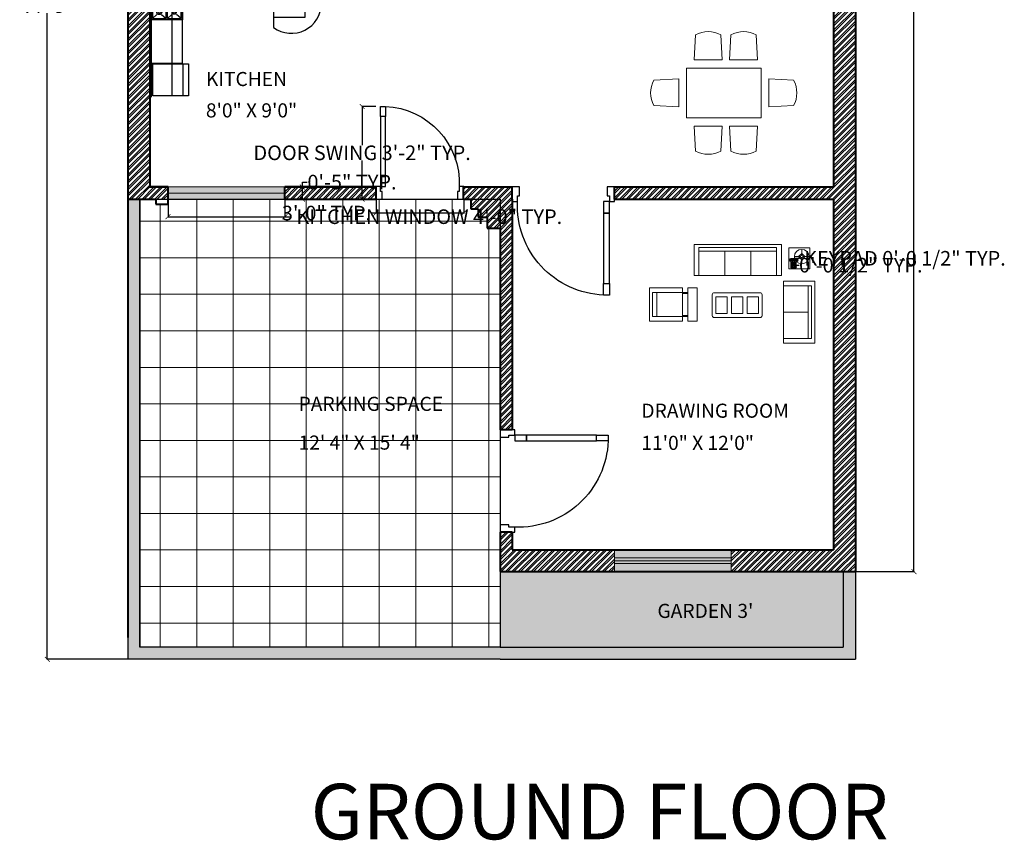
# Model space of a CAD drawing. Units: inches. Extents: x 528 to 2520, y -151 to 1354.
# Tile 1 of 41: x 542 to 947, y 706 to 1043. Entities that reach past the tile are written whole.
import ezdxf

# ---------------------------------------------------------------- set-up
doc = ezdxf.new("R2010")
doc.units = ezdxf.units.IN
doc.header["$MEASUREMENT"] = 0
for name, color, linetype, lineweight in [('A-ANNO-DIMS', 2, 'Continuous', 18), ('A-ANNO-TEXT', 7, 'Continuous', 30), ('A-AREA-IDEN', 7, 'Continuous', 18), ('A-Door', 150, 'Continuous', 25), ('A-FLOR-CASE', 11, 'Continuous', 20), ('A-FLOR-PATT', 7, 'Continuous', 13), ('A-FURN', 8, 'Continuous', 18), ('A-SITE-EDGE', 7, 'Continuous', 25), ('A-SITE-PATT', 7, 'Continuous', 13), ('A-WALL-PATT', 6, 'Continuous', 13), ('walls', 7, 'Continuous', 40), ('WINDOWS', 2, 'Continuous', 20)]:
    doc.layers.add(name, color=color, linetype=linetype, lineweight=lineweight)
doc.layers.add('A-GLAZ-PATT', color=152, linetype='Continuous', lineweight=13, true_color=0x2776bb)
doc.layers.add('L-PLNT-PATT', color=85, linetype='Continuous', lineweight=13, true_color=0x58ba48)
for name, color, linetype in [('ESYA', 11, 'Continuous'), ('NT', 1, 'Continuous'), ('TEFRIS', 11, 'Continuous')]:
    doc.layers.add(name, color=color, linetype=linetype)
doc.styles.get("Standard").update_dxf_attribs({"font": 'arial.ttf'})
doc.dimstyles.get("Standard").update_dxf_attribs({"dimtxt": 6, "dimasz": 2, "dimexe": 0.18, "dimexo": 0.0625, "dimgap": 0.09, "dimtad": 0, "dimtih": 1, "dimtoh": 1, "dimdec": 1, "dimzin": 0, "dimdsep": 46, "dimlunit": 3, "dimtxsty": 'Standard', "dimblk": 'ARCHTICK', "dimcen": 0.09, "dimadec": 0, "dimazin": 0, "dimtfac": 1, "dimtdec": 1, "dimtofl": 0, "dimtmove": 0, "dimatfit": 3, "dimfxl": 1, "dimtolj": 1, "dimtzin": 0, "dimarcsym": 0})

# ---------------------------------------------------------------- blocks, each defined once
blk = doc.blocks.new('A$C7DB75F4D')
at = {"layer": 'A-Door'}
for points in [[(625, 740), (625, 660), (665, 660), (665, 740)], [(625, 180), (625, 660), (665, 660), (665, 180)], [(625, 100), (625, 180), (665, 180), (665, 100)], [(35, 100), (35, 60), (50, 60), (50, 50), (50, 0), (0, 0), (0, 100)], [(665, 100), (700, 100), (700, 0), (650, 0), (650, 50), (650, 60), (665, 60)]]:
    blk.add_lwpolyline(points, close=True, dxfattribs=at)
at = {"layer": 'NT'}
blk.add_arc((650, 125), 615.5, 92.32782, 182.32782, dxfattribs=at)
blk = doc.blocks.new('AR365L')
blk.add_line((0, 0.1), (0.61, 0.1))
blk.add_lwpolyline([(0, 0), (0, 0.68), (0.61, 0.68), (0.61, 0)], close=True)
blk = doc.blocks.new('FIRIN1')
at = {"layer": 'ESYA'}
for p, q in [((0.288, -0.05), (0.288, -0.301)), ((0.398, -0.132), (0.312, -0.05)), ((0.575, -0.05), (0.489, -0.132)), ((0.288, -0.301), (0.025, -0.301)), ((0.025, -0.324), (0.111, -0.406)), ((0.202, -0.406), (0.288, -0.324)), ((0.398, -0.219), (0.312, -0.301)), ((0.398, -0.406), (0.312, -0.324)), ((0.575, -0.301), (0.489, -0.219)), ((0.575, -0.324), (0.489, -0.406)), ((0.025, -0.575), (0.111, -0.493)), ((0.202, -0.493), (0.288, -0.575)), ((0.398, -0.493), (0.312, -0.575)), ((0.575, -0.575), (0.489, -0.493))]:
    blk.add_line(p, q, dxfattribs=at)
blk.add_lwpolyline([(0, 0), (0.6, 0), (0.6, -0.6), (0, -0.6)], close=True, dxfattribs=at)
for points in [[(0.288, -0.05), (0.025, -0.05), (0.025, -0.301)], [(0.312, -0.05), (0.312, -0.301), (0.575, -0.301)], [(0.575, -0.301), (0.575, -0.05), (0.312, -0.05)], [(0.288, -0.575), (0.288, -0.324), (0.025, -0.324)], [(0.025, -0.324), (0.025, -0.575)], [(0.312, -0.575), (0.312, -0.324), (0.575, -0.324)], [(0.312, -0.575), (0.575, -0.575), (0.575, -0.324)], [(0.025, -0.575), (0.288, -0.575)]]:
    blk.add_lwpolyline(points, dxfattribs=at)
for centre, radius in [((0.156, -0.175), 0.0986), ((0.156, -0.175), 0.0936), ((0.444, -0.175), 0.0597), ((0.444, -0.175), 0.0294), ((0.156, -0.45), 0.0492), ((0.156, -0.45), 0.0242), ((0.444, -0.45), 0.0398), ((0.444, -0.45), 0.0196)]:
    blk.add_circle(centre, radius, dxfattribs=at)
blk = doc.blocks.new('ncvn')
for p, q in [((77868.4, -4466.7), (77868.4, -4520.7)), ((77949.4, -4466.7), (77868.4, -4466.7)), ((77949.4, -4520.7), (77949.4, -4466.7))]:
    blk.add_line(p, q)
at = {"layer": 'TEFRIS'}
for p, q in [((77783.7, -4466.7), (77783.7, -4763.4)), ((77783.7, -4466.7), (78049.5, -4466.7)), ((77902, -4516.6), (77902, -4471.6)), ((78049.5, -4466.7), (78049.5, -4553.6)), ((77819.7, -4502.8), (77819.7, -4759.2)), ((77819.7, -4502.8), (78049.5, -4502.8)), ((77837.7, -4520.8), (77837.7, -4704.7)), ((77837.7, -4520.8), (77995.5, -4520.8)), ((77868.4, -4520.7), (77949.4, -4520.7)), ((77995.5, -4520.8), (77995.5, -4643)), ((78049.5, -4555), (78049.5, -4625.7)), ((78049.5, -4625.7), (77995.8, -4625.7)), ((77783.7, -4704.7), (77837.7, -4704.7))]:
    blk.add_line(p, q, dxfattribs=at)
for points in [[(77868.4, -4466.7), (77868.4, -4520.7), (77949.4, -4520.7), (77949.4, -4466.7)], [(77871.4, -4471.6), (77871.4, -4516.6), (77947, -4516.6), (77947, -4471.6)]]:
    blk.add_lwpolyline(points, close=True, dxfattribs=at)
for points in [[(77911.5, -4488.6), (77925, -4475, -1), (77926.3, -4476.3), (77912.7, -4489.8, -1)], [(77906, -4486.7), (77906, -4507.2, 0.414214), (77911.4, -4512.6), (77937.6, -4512.6, 0.414214), (77943, -4507.2), (77943, -4486.7, 0.414214), (77937.6, -4481.3), (77911.4, -4481.3, 0.414214)], [(77906.5, -4486.7), (77906.5, -4507.2, 0.414214), (77911.4, -4512.1), (77937.6, -4512.1, 0.414214), (77942.4, -4507.2), (77942.4, -4486.7, 0.414214), (77937.6, -4481.9), (77911.4, -4481.9, 0.414214)], [(77913.5, -4476.3), (77919.7, -4476.3, -0.563183), (77919.7, -4477.4), (77913.5, -4477.4, -1)], [(77935.3, -4476.3), (77929.2, -4476.3, 0.563183), (77929.2, -4477.4), (77935.3, -4477.4, 1)]]:
    blk.add_lwpolyline(points, format="xyb", close=True, dxfattribs=at)
for points in [[(77873.2, -4477.9), (77900.2, -4477.9, -1), (77900.2, -4479.7), (77873.2, -4479.7, -1), (77873.2, -4477.9)], [(77873.2, -4480.6), (77900.2, -4480.6, -1), (77900.2, -4482.4), (77873.2, -4482.4, -1), (77873.2, -4480.6)], [(77873.2, -4483.3), (77900.2, -4483.3, -1), (77900.2, -4485.1), (77873.2, -4485.1, -1), (77873.2, -4483.3)], [(77873.2, -4486), (77900.2, -4486, -1), (77900.2, -4487.8), (77873.2, -4487.8, -1), (77873.2, -4486)], [(77873.2, -4488.7), (77900.2, -4488.7, -1), (77900.2, -4490.5), (77873.2, -4490.5, -1), (77873.2, -4488.7)], [(77873.2, -4491.4), (77900.2, -4491.4, -1), (77900.2, -4493.2), (77873.2, -4493.2, -1), (77873.2, -4491.4)], [(77873.2, -4494.1), (77900.2, -4494.1, -1), (77900.2, -4495.9), (77873.2, -4495.9, -1), (77873.2, -4494.1)], [(77873.2, -4496.8), (77900.2, -4496.8, -1), (77900.2, -4498.6), (77873.2, -4498.6, -1), (77873.2, -4496.8)], [(77873.2, -4499.5), (77900.2, -4499.5, -1), (77900.2, -4501.3), (77873.2, -4501.3, -1), (77873.2, -4499.5)], [(77873.2, -4502.2), (77900.2, -4502.2, -1), (77900.2, -4504), (77873.2, -4504, -1), (77873.2, -4502.2)], [(77873.2, -4504.9), (77900.2, -4504.9, -1), (77900.2, -4506.7), (77873.2, -4506.7, -1), (77873.2, -4504.9)], [(77873.2, -4507.6), (77900.2, -4507.6, -1), (77900.2, -4509.4), (77873.2, -4509.4, -1), (77873.2, -4507.6)], [(77873.2, -4510.3), (77900.2, -4510.3, -1), (77900.2, -4512.1), (77873.2, -4512.1, -1), (77873.2, -4510.3)]]:
    blk.add_lwpolyline(points, format="xyb", dxfattribs=at)
for points in [[(77901.2, -4520.7), (77901.2, -4521.6), (77902.1, -4521.6), (77902.1, -4520.7)], [(77915.6, -4520.7), (77915.6, -4521.6), (77916.5, -4521.6), (77916.5, -4520.7)]]:
    blk.add_lwpolyline(points, dxfattribs=at)
for centre, radius in [((77913, -4488.3), 0.571), ((77924.9, -4498.5), 2.86)]:
    blk.add_circle(centre, radius, dxfattribs=at)
for centre, radius, start, end in [((77918.7, -4476.9), 1.71, 199.4712, 160.5288), ((77924.4, -4476.9), 1.71, 75, 195), ((77930.2, -4476.9), 1.71, 19.4712, 340.5288), ((77924.4, -4476.9), 1.71, 255, 15), ((78026.2, -4601.3), 51.8, 233.6588, 63.2671)]:
    blk.add_arc(centre, radius, start, end, dxfattribs=at)
at = {"layer": 'TEFRIS', "xscale": 90, "yscale": 90, "zscale": 90}
blk.add_blockref('FIRIN1', (77783.8, -4575.9), dxfattribs=at)
at = {"layer": 'TEFRIS', "xscale": 90, "yscale": 90, "zscale": 90, "rotation": 90}
blk.add_blockref('AR365L', (77848.2, -4760.9), dxfattribs=at)
blk = doc.blocks.new('RECLIN32')
for p, q in [((16, 0), (16, -32)), ((-11.5, -3), (11.5, -3)), ((-11.5, -32), (-11.5, -3)), ((-11.5, -7), (11.5, -7)), ((11.5, -3), (11.5, -32)), ((-11.5, -32), (-11.5, -37)), ((-10.5, -32), (-10.5, -37)), ((10.5, -32), (10.5, -37)), ((11.5, -32), (11.5, -37))]:
    blk.add_line(p, q)
blk.add_lwpolyline([(16, -32), (-16, -32), (-16, 0), (16, 0)])
blk.add_lwpolyline([(-16, -46), (-16, -37), (16, -37), (16, -46)], close=True)
blk = doc.blocks.new('LOVESET5')
for p, q in [((35.75, 0), (35.75, -30.00001)), ((-19.75, -3), (31.25, -3)), ((-19.75, -30.00001), (-19.75, -3)), ((-19.75, -6.5), (31.25, -6.5)), ((5.75, -6.5), (5.75, -30.00001)), ((31.25, -3), (31.25, -30.00001))]:
    blk.add_line(p, q)
for points in [[(35.75, -30.00001), (-24.25, -30.00001), (-24.25, 0), (24.25, 0)], [(24.25, 0), (35.75, 0)]]:
    blk.add_lwpolyline(points)
blk = doc.blocks.new('TBLEN20S')
blk.add_lwpolyline([(-10, -10), (-10, 10), (10, 10), (10, -10)], close=True)
blk = doc.blocks.new('LAMP')
for p, q in [((-1, 0), (-7, 0)), ((0, 3), (-3, 0)), ((-3, 0), (0, -3)), ((0, 7), (0, 1)), ((3, 0), (0, 3)), ((0, -3), (3, 0)), ((1, 0), (7, 0)), ((0, -1), (0, -7))]:
    blk.add_line(p, q)
for radius in [7, 1]:
    blk.add_circle((0, 0), radius)
blk = doc.blocks.new('SOFA7')
for p, q in [((-37.5, -3), (37.5, -3)), ((-37.5, -30), (-37.5, -3)), ((-37.5, -6.5), (37.5, -6.5)), ((-12.5, -6.5), (-12.5, -30)), ((12.5, -6.5), (12.5, -30)), ((37.5, -3), (37.5, -30))]:
    blk.add_line(p, q)
blk.add_lwpolyline([(-42, -30), (-42, 0), (42, 0), (42, -30)], close=True)
blk = doc.blocks.new('TBLWGLAS')
for p, q in [((-22, 0), (22, 0)), ((-24, -22), (-24, -2)), ((-20.5, -20), (-20.5, -4)), ((-20.5, -4), (-9.5, -4)), ((-9.5, -4), (-9.5, -20)), ((-5.5, -20), (-5.5, -4)), ((-5.5, -4), (5.5, -4)), ((5.5, -4), (5.5, -20)), ((9.5, -20), (9.5, -4)), ((9.5, -4), (20.5, -4)), ((20.5, -4), (20.5, -20)), ((24, -2), (24, -22)), ((22, -24), (-22, -24)), ((-9.5, -20), (-20.5, -20)), ((5.5, -20), (-5.5, -20)), ((20.5, -20), (9.5, -20))]:
    blk.add_line(p, q)
for centre, start, end in [((-22, -2), 90, 180), ((22, -2), 0, 90), ((-22, -22), 180, 270), ((22, -22), 270, 0)]:
    blk.add_arc(centre, 2, start, end)
blk = doc.blocks.new('PHONE')
for p, q in [((-3.99, 3.5), (-3.99, 2.5)), ((4.01, 3.5), (-3.99, 3.5)), ((-3.99, 2.5), (4.01, 2.5)), ((-2.49, -4.03), (-2.49, 1.92)), ((-2.02, 4.5), (2.02, 4.5)), ((-1.99, 1), (-1.99, -4)), ((2.01, 1), (-1.99, 1)), ((-1.49, 4), (-0.74, 4)), ((-1.49, 3.5), (-1.49, 4)), ((-1.49, 2), (-1.49, 2.5)), ((-0.74, 2), (-1.49, 2)), ((1.01, 0.5), (-0.99, 0.5)), ((-0.99, 0.5), (-0.99, -3.5)), ((-0.74, 4), (-0.74, 3.5)), ((-0.74, 2.5), (-0.74, 2)), ((0.76, 4), (0.76, 3.5)), ((1.51, 4), (0.76, 4)), ((0.76, 2.5), (0.76, 2)), ((0.76, 2), (1.51, 2)), ((1.01, -3.5), (1.01, 0.5)), ((1.51, 3.5), (1.51, 4)), ((1.51, 2), (1.51, 2.5)), ((2.01, -4), (2.01, 1)), ((2.51, 1.95), (2.51, -4.06)), ((4.01, 2.5), (4.01, 3.5)), ((2.04, -4.5), (-2.01, -4.5)), ((-1.99, -4), (2.01, -4)), ((-0.99, -3.5), (1.01, -3.5))]:
    blk.add_line(p, q)
for centre, radius, start, end in [((-3.24, 3), 1.27, 24.02748, 336.6167), ((-2.05, 4.06), 0.442, 81.8699, 188.1301), ((2.07, 4.06), 0.442, 351.8699, 98.1301), ((3.26, 3), 1.25, 205.0096, 154.8206), ((-2.05, -4.06), 0.442, 171.8699, 278.1301), ((2.07, -4.06), 0.442, 261.8699, 8.1301)]:
    blk.add_arc(centre, radius, start, end)
blk = doc.blocks.new('table-20')
at = {"color": 0, "linetype": 'ByBlock'}
for p, q in [((-1.052, 0.533), (-1.074, 0.134)), ((-0.646, 0.533), (-0.624, 0.134)), ((-0.484, 0.533), (-0.506, 0.134)), ((-0.078, 0.533), (-0.056, 0.134)), ((-1.2, 0), (0, 0)), ((-1.2, -0.8), (-1.2, 0)), ((-0.624, 0.134), (-1.074, 0.134)), ((-0.056, 0.134), (-0.506, 0.134)), ((0, -0.8), (0, 0)), ((-1.723, -0.197), (-1.324, -0.175)), ((-1.324, -0.625), (-1.324, -0.175)), ((0.124, -0.625), (0.124, -0.175)), ((0.523, -0.197), (0.124, -0.175)), ((-1.723, -0.603), (-1.324, -0.625)), ((0.523, -0.603), (0.124, -0.625)), ((-1.2, -0.8), (0, -0.8)), ((-0.624, -0.934), (-1.074, -0.934)), ((-1.052, -1.333), (-1.074, -0.934)), ((-0.646, -1.333), (-0.624, -0.934)), ((-0.484, -1.333), (-0.506, -0.934)), ((-0.056, -0.934), (-0.506, -0.934)), ((-0.078, -1.333), (-0.056, -0.934))]:
    blk.add_line(p, q, dxfattribs=at)
for centre, start, end in [((-0.849, 0.159), 61.4891, 118.5109), ((-0.281, 0.159), 61.4891, 118.5109), ((-1.349, -0.4), 151.4891, 208.5109), ((0.149, -0.4), 331.4891, 28.5109), ((-0.849, -0.959), 241.4891, 298.5109), ((-0.281, -0.959), 241.4891, 298.5109)]:
    blk.add_arc(centre, 0.425, start, end, dxfattribs=at)
blk = doc.blocks.new('_ArchTick')
at = {"color": 0, "linetype": 'ByBlock', "const_width": 0.15}
blk.add_lwpolyline([(-0.5, -0.5), (0.5, 0.5)], dxfattribs=at)
blk = doc.blocks.new('*D24')
at = {"layer": 'A-ANNO-DIMS', "color": 0, "lineweight": -2, "transparency": 16777216}
for p, q in [((885.76, 1317.1), (909.9, 1317.1)), ((909.72, 1317.1), (909.72, 1069.76)), ((909.72, 816.1), (909.72, 1063.45)), ((885.76, 816.1), (909.9, 816.1))]:
    blk.add_line(p, q, dxfattribs=at)
at = {"layer": 'Defpoints', "color": 0, "transparency": 16777216}
for p in [(885.7, 1317.1), (885.7, 816.1), (909.72, 816.1)]:
    blk.add_point(p, dxfattribs=at)
at = {"layer": 'A-ANNO-DIMS', "color": 0, "lineweight": -2, "transparency": 16777216, "xscale": 2, "yscale": 2, "zscale": 2}
for p, rotation in [((909.72, 1317.1), 90), ((909.72, 816.1), 270)]:
    blk.add_blockref('_ArchTick', p, dxfattribs=dict(at, rotation=rotation))
at = {"layer": 'A-ANNO-DIMS', "color": 0, "transparency": 16777216, "insert": (909.72, 1066.6), "char_height": 6, "attachment_point": 5}
blk.add_mtext('\\A1;41\'-9.0"', dxfattribs=at)
blk = doc.blocks.new('WINDOW-48x5-PLAN')
for p, q in [((0, 5), (48, 5)), ((0, 2.5), (48, 2.5))]:
    blk.add_line(p, q)
blk.add_lwpolyline([(0, 5), (48, 5), (48, 0), (0, 0)], close=True)
blk = doc.blocks.new('WINDOW-48x9-PLAN')
for p, q in [((0, 5.63), (48, 5.63)), ((0, 4.5), (48, 4.5)), ((0, 3.37), (48, 3.37))]:
    blk.add_line(p, q)
blk.add_lwpolyline([(0, 9), (48, 9), (48, 0), (0, 0)], close=True)
blk = doc.blocks.new('TELEPHONE-KEYPAD')
for centre in [(0.05, 0.67), (0.07, 0.46), (0.09, 0.25), (0.1, 0.06), (0.26, 0.67), (0.27, 0.47), (0.27, 0.25), (0.29, 0.05), (0.48, 0.66), (0.48, 0.46), (0.49, 0.26), (0.5, 0.08)]:
    blk.add_circle(centre, 0.0493)
blk = doc.blocks.new('*D42')
at = {"layer": 'A-ANNO-DIMS', "color": 0, "lineweight": -2, "transparency": 16777216}
for p, q in [((688.64, 1007.18), (682.81, 1007.18)), ((682.99, 1007.18), (682.99, 991.34)), ((682.99, 969.1), (682.99, 984.94)), ((688.64, 969.1), (682.81, 969.1))]:
    blk.add_line(p, q, dxfattribs=at)
at = {"layer": 'Defpoints', "color": 0, "transparency": 16777216}
for p in [(682.99, 1007.18), (688.7, 1007.18), (688.7, 969.1)]:
    blk.add_point(p, dxfattribs=at)
at = {"layer": 'A-ANNO-DIMS', "color": 0, "lineweight": -2, "transparency": 16777216, "xscale": 2, "yscale": 2, "zscale": 2}
for p, rotation in [((682.99, 1007.18), 90), ((682.99, 969.1), 270)]:
    blk.add_blockref('_ArchTick', p, dxfattribs=dict(at, rotation=rotation))
at = {"layer": 'A-ANNO-DIMS', "color": 0, "transparency": 16777216, "insert": (682.99, 988.14), "char_height": 6, "attachment_point": 5}
blk.add_mtext('\\A1;DOOR SWING 3\'-2" TYP.', dxfattribs=at)
blk = doc.blocks.new('*D43')
at = {"layer": 'A-ANNO-DIMS', "color": 0, "lineweight": -2, "transparency": 16777216}
for p, q in [((688.7, 969.04), (688.7, 963.21)), ((724.72, 969.04), (724.72, 963.21)), ((688.7, 963.39), (686.7, 963.39)), ((724.72, 963.39), (688.7, 963.39))]:
    blk.add_line(p, q, dxfattribs=at)
at = {"layer": 'Defpoints', "color": 0, "transparency": 16777216}
for p in [(688.7, 969.1), (724.72, 969.1), (688.7, 963.39)]:
    blk.add_point(p, dxfattribs=at)
at = {"layer": 'A-ANNO-DIMS', "color": 0, "lineweight": -2, "transparency": 16777216, "xscale": 2, "yscale": 2, "zscale": 2, "rotation": 180}
blk.add_blockref('_ArchTick', (688.7, 963.39), dxfattribs=at)
at = {"layer": 'A-ANNO-DIMS', "color": 0, "lineweight": -2, "transparency": 16777216, "xscale": 2, "yscale": 2, "zscale": 2}
blk.add_blockref('_ArchTick', (724.72, 963.39), dxfattribs=at)
at = {"layer": 'A-ANNO-DIMS', "color": 0, "transparency": 16777216, "insert": (668.33, 963.39), "char_height": 6, "attachment_point": 5}
blk.add_mtext('\\A1;3\'-0" TYP.', dxfattribs=at)
blk = doc.blocks.new('*D76')
at = {"layer": 'A-ANNO-DIMS', "color": 0, "lineweight": -2, "transparency": 16777216}
for p, q in [((860.61, 942.81), (860.83, 942.81)), ((860.65, 942.81), (860.65, 944.81)), ((860.65, 944.81), (862.65, 944.81)), ((860.65, 942.09), (860.65, 942.81)), ((860.61, 942.09), (860.83, 942.09))]:
    blk.add_line(p, q, dxfattribs=at)
at = {"layer": 'Defpoints', "color": 0, "transparency": 16777216}
for p in [(860.54, 942.81), (860.65, 942.81), (860.54, 942.09)]:
    blk.add_point(p, dxfattribs=at)
at = {"layer": 'A-ANNO-DIMS', "color": 0, "lineweight": -2, "transparency": 16777216, "xscale": 2, "yscale": 2, "zscale": 2}
for p, rotation in [((860.65, 942.81), 90), ((860.65, 942.09), 270)]:
    blk.add_blockref('_ArchTick', p, dxfattribs=dict(at, rotation=rotation))
at = {"layer": 'A-ANNO-DIMS', "color": 0, "transparency": 16777216, "insert": (906.05, 944.81), "char_height": 6, "attachment_point": 5}
blk.add_mtext('\\A1;KEYPAD 0\'-0 1/2" TYP.', dxfattribs=at)
blk = doc.blocks.new('*D77')
at = {"layer": 'A-ANNO-DIMS', "color": 0, "lineweight": -2, "transparency": 16777216}
for p, q in [((860, 942.03), (860, 941.8)), ((860, 941.98), (860.54, 941.98)), ((860.54, 942.03), (860.54, 941.8)), ((860.54, 941.98), (862.54, 941.98))]:
    blk.add_line(p, q, dxfattribs=at)
at = {"layer": 'Defpoints', "color": 0, "transparency": 16777216}
for p in [(860, 942.09), (860.54, 942.09), (860.54, 941.98)]:
    blk.add_point(p, dxfattribs=at)
at = {"layer": 'A-ANNO-DIMS', "color": 0, "lineweight": -2, "transparency": 16777216, "xscale": 2, "yscale": 2, "zscale": 2, "rotation": 180}
blk.add_blockref('_ArchTick', (860, 941.98), dxfattribs=at)
at = {"layer": 'A-ANNO-DIMS', "color": 0, "lineweight": -2, "transparency": 16777216, "xscale": 2, "yscale": 2, "zscale": 2}
blk.add_blockref('_ArchTick', (860.54, 941.98), dxfattribs=at)
at = {"layer": 'A-ANNO-DIMS', "color": 0, "transparency": 16777216, "insert": (887.91, 941.98), "char_height": 6, "attachment_point": 5}
blk.add_mtext('\\A1;0\'-0 1/2" TYP.', dxfattribs=at)
blk = doc.blocks.new('*D84')
at = {"layer": 'A-ANNO-DIMS', "color": 0, "lineweight": -2, "transparency": 16777216}
for p, q in [((603.24, 969.04), (603.24, 961.72)), ((651.24, 969.04), (651.24, 961.72)), ((603.24, 961.9), (651.24, 961.9)), ((651.24, 961.9), (653.24, 961.9))]:
    blk.add_line(p, q, dxfattribs=at)
at = {"layer": 'Defpoints', "color": 0, "transparency": 16777216}
for p in [(603.24, 969.1), (651.24, 969.1), (651.24, 961.9)]:
    blk.add_point(p, dxfattribs=at)
at = {"layer": 'A-ANNO-DIMS', "color": 0, "lineweight": -2, "transparency": 16777216, "xscale": 2, "yscale": 2, "zscale": 2, "rotation": 180}
blk.add_blockref('_ArchTick', (603.24, 961.9), dxfattribs=at)
at = {"layer": 'A-ANNO-DIMS', "color": 0, "lineweight": -2, "transparency": 16777216, "xscale": 2, "yscale": 2, "zscale": 2}
blk.add_blockref('_ArchTick', (651.24, 961.9), dxfattribs=at)
at = {"layer": 'A-ANNO-DIMS', "color": 0, "transparency": 16777216, "insert": (710.6, 961.9), "char_height": 6, "attachment_point": 5}
blk.add_mtext('\\A1;KITCHEN WINDOW 4\'-0" TYP.', dxfattribs=at)
blk = doc.blocks.new('*D85')
at = {"layer": 'A-ANNO-DIMS', "color": 0, "lineweight": -2, "transparency": 16777216}
for p, q in [((658.44, 974.1), (658.44, 976.1)), ((658.44, 976.1), (660.44, 976.1)), ((651.31, 974.1), (658.62, 974.1)), ((658.44, 969.1), (658.44, 974.1)), ((651.31, 969.1), (658.62, 969.1))]:
    blk.add_line(p, q, dxfattribs=at)
at = {"layer": 'Defpoints', "color": 0, "transparency": 16777216}
for p in [(651.24, 974.1), (658.44, 974.1), (651.24, 969.1)]:
    blk.add_point(p, dxfattribs=at)
at = {"layer": 'A-ANNO-DIMS', "color": 0, "lineweight": -2, "transparency": 16777216, "xscale": 2, "yscale": 2, "zscale": 2}
for p, rotation in [((658.44, 974.1), 90), ((658.44, 969.1), 270)]:
    blk.add_blockref('_ArchTick', p, dxfattribs=dict(at, rotation=rotation))
at = {"layer": 'A-ANNO-DIMS', "color": 0, "transparency": 16777216, "insert": (678.82, 976.1), "char_height": 6, "attachment_point": 5}
blk.add_mtext('\\A1;0\'-5" TYP.', dxfattribs=at)
blk = doc.blocks.new('*D92')
at = {"layer": 'A-ANNO-DIMS', "color": 0, "lineweight": -2, "transparency": 16777216}
for p, q in [((586.63, 1317.1), (553.42, 1317.1)), ((553.6, 1317.1), (553.6, 1051.76)), ((553.6, 780.1), (553.6, 1045.45)), ((586.63, 780.1), (553.42, 780.1))]:
    blk.add_line(p, q, dxfattribs=at)
at = {"layer": 'Defpoints', "color": 0, "transparency": 16777216}
for p in [(553.6, 1317.1), (586.7, 1317.1), (586.7, 780.1)]:
    blk.add_point(p, dxfattribs=at)
at = {"layer": 'A-ANNO-DIMS', "color": 0, "lineweight": -2, "transparency": 16777216, "xscale": 2, "yscale": 2, "zscale": 2}
for p, rotation in [((553.6, 1317.1), 90), ((553.6, 780.1), 270)]:
    blk.add_blockref('_ArchTick', p, dxfattribs=dict(at, rotation=rotation))
at = {"layer": 'A-ANNO-DIMS', "color": 0, "transparency": 16777216, "insert": (553.6, 1048.6), "char_height": 6, "attachment_point": 5}
blk.add_mtext('\\A1;44\'-9"', dxfattribs=at)

msp = doc.modelspace()

# ---------------------------------------------------------------- hatches: boundary and pattern name
at = {"layer": 'A-FLOR-PATT', "transparency": 33554523}
h = msp.add_hatch(dxfattribs=at)
h.set_pattern_fill('NET', color=256, scale=120)
h.paths.add_polyline_path([(739.7, 957.24), (734.43, 957.24), (734.43, 961.68), (730.74, 961.68), (730.74, 965.12), (727.7, 965.12), (727.7, 969.1), (603.24, 969.1), (603.24, 967.1), (598.24, 967.1), (598.24, 969.1), (591.7, 969.1), (591.7, 785.1), (739.7, 785.1)])
at = {"layer": 'A-GLAZ-PATT'}
h = msp.add_hatch(color=256, dxfattribs=at)
h.dxf.hatch_style = 1
h.paths.add_polyline_path([(651.24, 974.1), (603.24, 974.1), (603.24, 971.6), (651.24, 971.6)])
h.paths.add_polyline_path([(651.24, 971.6), (603.24, 971.6), (603.24, 969.1), (651.24, 969.1)])
h = msp.add_hatch(color=256, dxfattribs=at)
h.dxf.hatch_style = 1
h.paths.add_polyline_path([(834.7, 825.1), (786.7, 825.1), (786.7, 821.73), (834.7, 821.73)])
h.paths.add_polyline_path([(834.7, 821.73), (786.7, 821.73), (786.7, 820.6), (834.7, 820.6)])
h.paths.add_polyline_path([(834.7, 820.6), (786.7, 820.6), (786.7, 819.47), (834.7, 819.47)])
h.paths.add_polyline_path([(834.7, 819.47), (786.7, 819.47), (786.7, 816.1), (834.7, 816.1)])
at = {"layer": 'A-SITE-PATT'}
h = msp.add_hatch(color=256, dxfattribs=at)
h.dxf.hatch_style = 1
h.paths.add_polyline_path([(885.7, 816.1), (880.7, 816.1), (880.7, 785.1), (739.7, 785.1), (591.7, 785.1), (591.7, 969.1), (586.7, 969.1), (586.7, 789.1), (586.7, 780.1), (739.7, 780.1), (885.7, 780.1)])
at = {"layer": 'A-WALL-PATT'}
h = msp.add_hatch(dxfattribs=at)
h.set_pattern_fill('ANSI32', color=256, scale=5)
h.paths.add_polyline_path([(595.7, 1163.86), (586.7, 1163.86), (586.7, 969.1), (598.24, 969.1), (603.24, 969.1), (603.24, 974.1), (595.7, 974.1), (595.7, 1082.1), (691.7, 1082.1), (691.7, 1087.1), (691.7, 1106.1), (697.7, 1106.1), (697.7, 1111.1), (686.7, 1111.1), (686.7, 1087.1), (595.7, 1087.1)])
h.paths.add_polyline_path([(688.7, 974.1), (651.24, 974.1), (651.24, 969.1), (688.7, 969.1)])
h.paths.add_polyline_path([(885.7, 1171.37), (876.7, 1171.37), (876.7, 1111.1), (786.7, 1111.1), (786.7, 1106.1), (876.7, 1106.1), (876.7, 974.1), (786.7, 974.1), (786.7, 969.1), (876.7, 969.1), (876.7, 825.1), (834.7, 825.1), (834.7, 816.1), (885.7, 816.1)])
h.paths.add_polyline_path([(885.7, 1317.1), (876.65, 1317.1), (876.65, 1308.1), (876.7, 1308.1), (876.7, 1248.1), (822.7, 1248.1), (822.7, 1243.1), (876.7, 1243.1), (876.7, 1219.37), (885.7, 1219.37)])
h.paths.add_polyline_path([(852.65, 1317.1), (787.7, 1317.1), (787.7, 1248.1), (784.26, 1248.1), (784.26, 1243.1), (792.7, 1243.1), (792.7, 1249.1), (792.7, 1308.1), (852.65, 1308.1)])
h.paths.add_polyline_path([(684.7, 1317.1), (619.7, 1317.1), (619.7, 1308.1), (679.7, 1308.1), (679.7, 1248.1), (679.7, 1243.1), (684.7, 1243.1), (684.7, 1248.25)])
h.paths.add_polyline_path([(595.7, 1308.1), (595.7, 1317.1), (586.7, 1317.1), (586.7, 1211.86), (595.7, 1211.86), (595.7, 1243.1), (649.7, 1243.1), (649.7, 1248.1), (595.7, 1248.1)])
h.paths.add_polyline_path([(744.7, 969.1), (744.7, 974.1), (724.7, 974.1), (724.7, 969.1), (739.7, 969.1), (739.7, 874.29), (744.7, 874.29)])
h.paths.add_polyline_path([(739.7, 969.1), (727.7, 969.1), (727.7, 965.12), (730.74, 965.12), (730.74, 961.68), (734.43, 961.68), (734.43, 957.24), (739.7, 957.24)], flags=17)
h.paths.add_polyline_path([(786.7, 825.1), (744.7, 825.1), (744.7, 832.29), (739.7, 832.29), (739.7, 816.1), (786.7, 816.1)])
at = {"layer": 'L-PLNT-PATT', "transparency": 33554577}
h = msp.add_hatch(color=256, dxfattribs=at)
h.dxf.hatch_style = 1
h.paths.add_polyline_path([(880.7, 816.1), (739.7, 816.1), (739.7, 785.1), (880.7, 785.1)])
h.paths.add_polyline_path([(802.83, 795.49), (848.74, 795.49), (848.74, 804.48), (802.83, 804.48)], flags=24)

# ---------------------------------------------------------------- linework, layer by layer
at = {"layer": 'A-SITE-EDGE'}
for p, q in [((591.7, 969.1), (591.7, 785.1)), ((739.7, 816.1), (739.7, 785.1)), ((880.7, 816.1), (880.7, 785.1)), ((885.7, 816.1), (885.7, 780.1)), ((586.7, 789.1), (586.7, 780.1)), ((739.7, 785.1), (591.7, 785.1)), ((739.7, 785.1), (880.7, 785.1)), ((739.7, 780.1), (586.7, 780.1)), ((739.7, 780.1), (885.7, 780.1))]:
    msp.add_line(p, q, dxfattribs=at)
msp.add_lwpolyline([(591.7, 969.1), (739.7, 969.1), (739.7, 785.1), (591.7, 785.1)], close=True, dxfattribs=at)
at = {"layer": 'walls'}
for p, q in [((586.7, 1317.1), (586.7, 789.1)), ((885.7, 1317.1), (885.7, 816.1)), ((876.7, 1106.1), (876.7, 974.1)), ((595.7, 1082.1), (595.7, 974.1)), ((595.7, 974.1), (603.24, 974.1)), ((603.24, 974.1), (595.7, 974.1)), ((603.24, 967.1), (603.24, 974.1)), ((688.7, 974.1), (651.24, 974.1)), ((651.24, 969.1), (651.24, 974.1)), ((651.24, 974.1), (688.7, 974.1)), ((688.7, 969.1), (688.7, 974.1)), ((724.7, 969.1), (724.7, 974.1)), ((724.7, 974.1), (744.7, 974.1)), ((744.7, 969.1), (744.7, 974.1)), ((786.7, 969.1), (786.7, 974.1)), ((786.7, 974.1), (876.7, 974.1)), ((586.7, 969.1), (598.24, 969.1)), ((598.24, 969.1), (598.24, 967.1)), ((598.24, 967.1), (603.24, 967.1)), ((651.24, 969.1), (688.7, 969.1)), ((724.7, 969.1), (727.7, 969.1)), ((727.7, 969.1), (727.7, 965.12)), ((744.7, 969.1), (744.7, 874.29)), ((786.7, 969.1), (876.7, 969.1)), ((876.7, 969.1), (876.7, 825.1)), ((727.7, 965.12), (730.74, 965.12)), ((730.74, 965.12), (730.74, 961.68)), ((730.74, 961.68), (734.43, 961.68)), ((734.43, 961.68), (734.43, 957.24)), ((734.43, 957.24), (739.7, 957.24)), ((739.7, 957.24), (739.7, 874.29)), ((744.7, 874.29), (739.7, 874.29)), ((744.7, 832.29), (739.7, 832.29)), ((739.7, 832.29), (739.7, 816.1)), ((744.7, 832.29), (744.7, 825.1)), ((744.7, 825.1), (876.7, 825.1)), ((739.7, 816.1), (885.7, 816.1))]:
    msp.add_line(p, q, dxfattribs=at)

# ---------------------------------------------------------------- block references
at = {"layer": 'A-Door', "xscale": -0.0514539602427209, "yscale": 0.0514539602427209, "zscale": 0.0514539602427209}
msp.add_blockref('A$C7DB75F4D', (724.72, 969.1), dxfattribs=at)
at = {"layer": 'A-Door', "xscale": -0.0600000000000059, "yscale": 0.0600000000000059, "zscale": 0.0600000000000059}
for p, rotation in [((744.7, 974.1), 180), ((739.7, 832.29), 270)]:
    msp.add_blockref('A$C7DB75F4D', p, dxfattribs=dict(at, rotation=rotation))
at = {"layer": 'A-FLOR-CASE', "xscale": 0.2377471155606993, "yscale": 0.2377471155606993, "zscale": 0.2377471155606993}
msp.add_blockref('ncvn', (-17896.58, 2143.47), dxfattribs=at)
at = {"layer": 'A-FURN', "xscale": 25.57841077690889, "yscale": 25.57841077690889, "zscale": 25.57841077690889}
msp.add_blockref('table-20', (846.93, 1022.96), dxfattribs=at)
at = {"layer": 'A-FURN', "extrusion": (0, 0, -1), "xscale": 0.4266539259093383, "yscale": 0.4266539259093383, "zscale": -0.426653925909338}
for name, p in [('SOFA7', (-837.33, 950.48)), ('TBLEN20S', (-862.66, 944.79)), ('LAMP', (-863.61, 945.5)), ('PHONE', (-860.25, 942.81)), ('TBLWGLAS', (-837.09, 930.69))]:
    msp.add_blockref(name, p, dxfattribs=at)
at = {"layer": 'A-FURN'}
msp.add_blockref('TELEPHONE-KEYPAD', (860, 942.09), dxfattribs=at)
at = {"layer": 'A-FURN', "extrusion": (0, 0, -1), "xscale": 0.4266539259093436, "yscale": 0.4266539259093436, "zscale": -0.426653925909338}
for name, p, rotation in [('LOVESET5', (-868.98, 920.23), 89.99999999999947), ('RECLIN32', (-801.04, 925.82), 269.9999999999994)]:
    msp.add_blockref(name, p, dxfattribs=dict(at, rotation=rotation))
at = {"layer": 'WINDOWS'}
for name, p in [('WINDOW-48x5-PLAN', (603.24, 969.1)), ('WINDOW-48x9-PLAN', (786.7, 816.1))]:
    msp.add_blockref(name, p, dxfattribs=at)

# ---------------------------------------------------------------- texts
at = {"layer": 'A-ANNO-TEXT'}
msp.add_text('GROUND FLOOR', height=22.7949, dxfattribs=at).set_placement((661.86, 706.16))
at = {"layer": 'A-AREA-IDEN'}
for s, height, p in [('KITCHEN', 5.793, (618.8, 1015.55)), ('8\'0" X 9\'0"', 5.7926, (618.8, 1002.67)), ('PARKING SPACE', 5.7926, (656.88, 882.13)), ('DRAWING ROOM', 5.7926, (797.73, 879.32)), ('12\' 4" X 15\' 4"', 5.7926, (656.88, 866.21)), ('11\'0" X 12\'0"', 5.7926, (797.73, 866.1)), ("GARDEN 3'", 5.793, (804.33, 797.09))]:
    msp.add_text(s, height=height, dxfattribs=at).set_placement(p)

# ---------------------------------------------------------------- dimensions: what is measured, and where the dimension line sits
at = {"layer": 'A-ANNO-DIMS'}
for base, p1, p2, override, picture, middle in [((553.6, 1317.1), (586.7, 780.1), (586.7, 1317.1), {"dimdec": 1, "dimlfac": 1, "dimrnd": 0, "dimzin": 1, "dimdsep": 46, "dimlunit": 4, "dimfrac": 2}, '*D92', (553.6, 1048.6)), ((909.72, 816.1), (885.7, 1317.1), (885.7, 816.1), {"dimclrd": 0, "dimclre": 0, "dimclrt": 0}, '*D24', (909.72, 1066.6))]:
    dim = msp.add_linear_dim(base=base, p1=p1, p2=p2, angle=90, dimstyle='Standard', override=override, dxfattribs=at)
    dim.commit()
    dim.dimension.update_dxf_attribs({"geometry": picture, "text_midpoint": middle})
for base, p1, p2, angle, text, picture, middle in [((682.99, 1007.18), (688.7, 969.1), (688.7, 1007.18), 90, 'DOOR SWING <> TYP.', '*D42', (682.99, 988.14)), ((658.44, 974.1), (651.24, 969.1), (651.24, 974.1), 90, '<> TYP.', '*D85', (678.82, 976.1)), ((688.7, 963.39), (724.72, 969.1), (688.7, 969.1), 180, '<> TYP.', '*D43', (668.33, 963.39)), ((860.65, 942.81), (860.54, 942.09), (860.54, 942.81), 90, 'KEYPAD <> TYP.', '*D76', (906.05, 944.81))]:
    dim = msp.add_linear_dim(base=base, p1=p1, p2=p2, angle=angle, text=text, dimstyle='Standard', override={"dimdec": 1, "dimlfac": 1, "dimrnd": 0, "dimzin": 1, "dimdsep": 46, "dimlunit": 4, "dimfrac": 2}, dxfattribs=at)
    dim.commit()
    dim.dimension.update_dxf_attribs({"geometry": picture, "text_midpoint": middle})
for base, p1, p2, text, picture, middle in [((651.24, 961.9), (603.24, 969.1), (651.24, 969.1), 'KITCHEN WINDOW <> TYP.', '*D84', (710.6, 961.9)), ((860.54, 941.98), (860, 942.09), (860.54, 942.09), '<> TYP.', '*D77', (887.91, 941.98))]:
    dim = msp.add_linear_dim(base=base, p1=p1, p2=p2, text=text, dimstyle='Standard', override={"dimdec": 1, "dimlfac": 1, "dimrnd": 0, "dimzin": 1, "dimdsep": 46, "dimlunit": 4, "dimfrac": 2}, dxfattribs=at)
    dim.commit()
    dim.dimension.update_dxf_attribs({"geometry": picture, "text_midpoint": middle})

doc.saveas('drawing.dxf')
